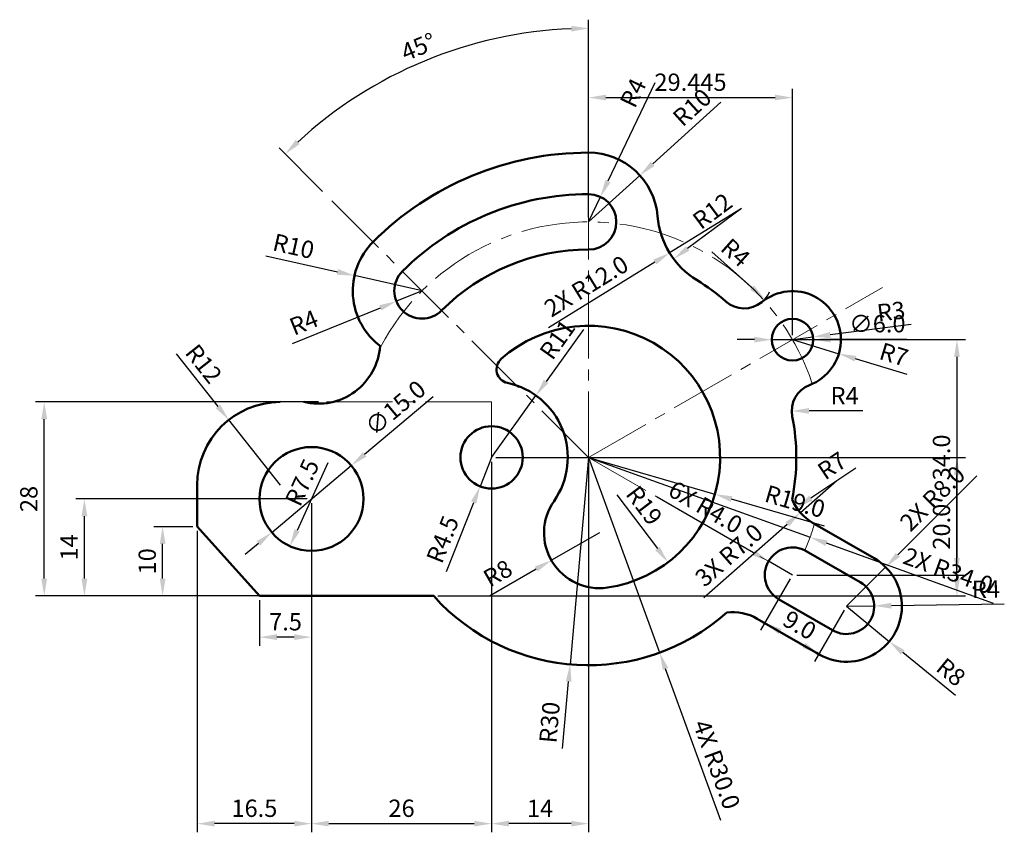
# Model space of a CAD drawing. Units: millimetres. Extents: x 1693 to 1835, y 1183 to 1300.
import ezdxf

# ---------------------------------------------------------------- set-up
doc = ezdxf.new("R2010")
doc.units = ezdxf.units.MM
doc.linetypes.add('CENTER2', pattern=[28.575, 19.05, -3.175, 3.175, -3.175])
for name, color, linetype, lineweight in [('M-CNTR', 4, 'CENTER2', 18), ('M-DIMS', 2, 'Continuous', 25), ('M-OUTL', 7, 'Continuous', 50)]:
    doc.layers.add(name, color=color, linetype=linetype, lineweight=lineweight)
doc.styles.get("Standard").update_dxf_attribs({"font": 'arial.ttf'})
doc.dimstyles.new('ISO-25', dxfattribs={"dimtxt": 2.5, "dimasz": 2.5, "dimexe": 1.25, "dimexo": 0.625, "dimtad": 1, "dimdsep": 46, "dimtxsty": 'Standard', "dimcen": 2.5, "dimadec": 0, "dimazin": 0, "dimtfac": 1, "dimtmove": 0, "dimatfit": 3, "dimfxl": 1, "dimarcsym": 0})

# ---------------------------------------------------------------- blocks, each defined once
blk = doc.blocks.new('*D1')
at = {"layer": 'Defpoints', "color": 0, "ltscale": 0.5, "transparency": 16777216}
for p in [(1759.38, 1296.69), (1775.41, 1275.52), (1737.44, 1274.82), (1775.41, 1236.85), (1775.41, 1236.85)]:
    blk.add_point(p, dxfattribs=at)
at = {"layer": 'M-DIMS', "color": 0, "lineweight": -2, "ltscale": 0.5, "transparency": 16777216}
for p, q in [((1775.41, 1276.15), (1775.41, 1300.05)), ((1737, 1275.26), (1730.72, 1281.54))]:
    blk.add_line(p, q, dxfattribs=at)
blk.add_arc((1775.41, 1236.85), 61.94, 92.3125, 132.6875, dxfattribs=at)
at = {"layer": 'M-DIMS', "color": 0, "ltscale": 0.5, "transparency": 16777216}
for points in [[(1772.9, 1299.16), (1772.92, 1298.33), (1775.41, 1298.8)], [(1733.7, 1282.09), (1733.12, 1282.69), (1731.61, 1280.65)]]:
    blk.add_solid(points, dxfattribs=at)
at = {"layer": 'M-DIMS', "color": 0, "ltscale": 0.5, "transparency": 16777216, "insert": (1750.98, 1295.83), "char_height": 2.5, "attachment_point": 5, "rotation": 22.5}
blk.add_mtext('45°', dxfattribs=at)
blk = doc.blocks.new('*D2')
at = {"layer": 'Defpoints', "color": 0, "transparency": 16777216}
for p in [(1777.13, 1274.46), (1775.41, 1270.85)]:
    blk.add_point(p, dxfattribs=at)
at = {"layer": 'M-DIMS', "color": 0, "lineweight": -2, "transparency": 16777216}
for p, q in [((1784.96, 1290.92), (1778.2, 1276.72)), ((1775.41, 1270.85), (1777.13, 1274.46))]:
    blk.add_line(p, q, dxfattribs=at)
at = {"layer": 'M-DIMS', "color": 0, "transparency": 16777216}
blk.add_solid([(1777.83, 1276.9), (1778.58, 1276.54), (1777.13, 1274.46)], dxfattribs=at)
at = {"layer": 'M-DIMS', "color": 0, "transparency": 16777216, "insert": (1782.13, 1289.34), "char_height": 2.5, "attachment_point": 5, "rotation": 64.5408}
blk.add_mtext('R4', dxfattribs=at)
blk = doc.blocks.new('*D3')
at = {"layer": 'Defpoints', "color": 0, "transparency": 16777216}
for p in [(1782.82, 1277.57), (1775.41, 1270.85)]:
    blk.add_point(p, dxfattribs=at)
at = {"layer": 'M-DIMS', "color": 0, "lineweight": -2, "transparency": 16777216}
for p, q in [((1794.52, 1288.16), (1784.67, 1279.24)), ((1775.41, 1270.85), (1782.82, 1277.57))]:
    blk.add_line(p, q, dxfattribs=at)
at = {"layer": 'M-DIMS', "color": 0, "transparency": 16777216}
blk.add_solid([(1784.39, 1279.55), (1784.95, 1278.93), (1782.82, 1277.57)], dxfattribs=at)
at = {"layer": 'M-DIMS', "color": 0, "transparency": 16777216, "insert": (1790.57, 1287.15), "char_height": 2.5, "attachment_point": 5, "rotation": 42.1642}
blk.add_mtext('R10', dxfattribs=at)
blk = doc.blocks.new('*D4')
at = {"layer": 'Defpoints', "color": 0, "transparency": 16777216}
for p in [(1804.85, 1253.85), (1811.55, 1251.82)]:
    blk.add_point(p, dxfattribs=at)
at = {"layer": 'M-DIMS', "color": 0, "lineweight": -2, "transparency": 16777216}
for p, q in [((1804.85, 1253.85), (1811.55, 1251.82)), ((1821.39, 1248.84), (1813.94, 1251.1))]:
    blk.add_line(p, q, dxfattribs=at)
at = {"layer": 'M-DIMS', "color": 0, "transparency": 16777216}
blk.add_solid([(1814.07, 1251.5), (1813.82, 1250.7), (1811.55, 1251.82)], dxfattribs=at)
at = {"layer": 'M-DIMS', "color": 0, "transparency": 16777216, "insert": (1819.41, 1251.4), "char_height": 2.5, "attachment_point": 5, "rotation": 343.1414}
blk.add_mtext('R7', dxfattribs=at)
blk = doc.blocks.new('*D5')
at = {"layer": 'Defpoints', "color": 0, "transparency": 16777216}
for p in [(1807.83, 1254.24), (1804.85, 1253.85)]:
    blk.add_point(p, dxfattribs=at)
at = {"layer": 'M-DIMS', "color": 0, "lineweight": -2, "transparency": 16777216}
for p, q in [((1821.99, 1256.06), (1810.31, 1254.56)), ((1804.85, 1253.85), (1807.83, 1254.24))]:
    blk.add_line(p, q, dxfattribs=at)
at = {"layer": 'M-DIMS', "color": 0, "transparency": 16777216}
blk.add_solid([(1810.25, 1254.97), (1810.36, 1254.14), (1807.83, 1254.24)], dxfattribs=at)
at = {"layer": 'M-DIMS', "color": 0, "transparency": 16777216, "insert": (1819.13, 1257.61), "char_height": 2.5, "attachment_point": 5, "rotation": 7.341}
blk.add_mtext('R3', dxfattribs=at)
blk = doc.blocks.new('*D6')
at = {"layer": 'Defpoints', "color": 0, "transparency": 16777216}
for p in [(1797.33, 1272.68), (1787.7, 1265.51)]:
    blk.add_point(p, dxfattribs=at)
at = {"layer": 'M-DIMS', "color": 0, "lineweight": -2, "transparency": 16777216}
blk.add_line((1797.49, 1272.79), (1789.71, 1267.01), dxfattribs=at)
at = {"layer": 'M-DIMS', "color": 0, "transparency": 16777216}
blk.add_solid([(1789.46, 1267.34), (1789.96, 1266.67), (1787.7, 1265.51)], dxfattribs=at)
at = {"layer": 'M-DIMS', "color": 0, "transparency": 16777216, "insert": (1793.48, 1272.16), "char_height": 2.5, "attachment_point": 5, "rotation": 36.6408}
blk.add_mtext('R12', dxfattribs=at)
blk = doc.blocks.new('*D7')
at = {"layer": 'Defpoints', "color": 0, "transparency": 16777216}
for p in [(1797.88, 1262.36), (1800.87, 1259.7)]:
    blk.add_point(p, dxfattribs=at)
at = {"layer": 'M-DIMS', "color": 0, "lineweight": -2, "transparency": 16777216}
blk.add_line((1793.21, 1266.54), (1799, 1261.36), dxfattribs=at)
blk.add_arc((1797.88, 1262.36), 4, 309.3093, 336.1142, dxfattribs=at)
at = {"layer": 'M-DIMS', "color": 0, "transparency": 16777216}
blk.add_solid([(1799.28, 1261.67), (1798.73, 1261.05), (1800.87, 1259.7)], dxfattribs=at)
at = {"layer": 'M-DIMS', "color": 0, "transparency": 16777216, "insert": (1796.42, 1266.18), "char_height": 2.5, "attachment_point": 5, "rotation": 318.2093}
blk.add_mtext('R4', dxfattribs=at)
blk = doc.blocks.new('*D8')
at = {"layer": 'Defpoints', "color": 0, "transparency": 16777216}
for p in [(1804.74, 1243.56), (1808.74, 1243.56)]:
    blk.add_point(p, dxfattribs=at)
at = {"layer": 'M-DIMS', "color": 0, "lineweight": -2, "transparency": 16777216}
blk.add_line((1815.01, 1243.56), (1807.24, 1243.56), dxfattribs=at)
at = {"layer": 'M-DIMS', "color": 0, "transparency": 16777216}
blk.add_solid([(1807.24, 1243.98), (1807.24, 1243.15), (1804.74, 1243.56)], dxfattribs=at)
at = {"layer": 'M-DIMS', "color": 0, "transparency": 16777216, "insert": (1812.38, 1245.44), "char_height": 2.5, "attachment_point": 5}
blk.add_mtext('R4', dxfattribs=at)
blk = doc.blocks.new('*D9')
at = {"layer": 'Defpoints', "color": 0, "transparency": 16777216}
for p in [(1811.25, 1233.48), (1805.44, 1229.58)]:
    blk.add_point(p, dxfattribs=at)
at = {"layer": 'M-DIMS', "color": 0, "lineweight": -2, "transparency": 16777216}
blk.add_line((1813.98, 1235.31), (1807.51, 1230.97), dxfattribs=at)
at = {"layer": 'M-DIMS', "color": 0, "transparency": 16777216}
blk.add_solid([(1807.28, 1231.32), (1807.74, 1230.63), (1805.44, 1229.58)], dxfattribs=at)
at = {"layer": 'M-DIMS', "color": 0, "transparency": 16777216, "insert": (1810.74, 1235.39), "char_height": 2.5, "attachment_point": 5, "rotation": 33.8392}
blk.add_mtext('R7', dxfattribs=at)
blk = doc.blocks.new('*D10')
at = {"layer": 'Defpoints', "color": 0, "transparency": 16777216}
for p in [(1812.65, 1215.35), (1816.65, 1215.41)]:
    blk.add_point(p, dxfattribs=at)
at = {"layer": 'M-DIMS', "color": 0, "lineweight": -2, "transparency": 16777216}
for p, q in [((1835.44, 1215.66), (1819.15, 1215.44)), ((1812.65, 1215.35), (1816.65, 1215.41))]:
    blk.add_line(p, q, dxfattribs=at)
at = {"layer": 'M-DIMS', "color": 0, "transparency": 16777216}
blk.add_solid([(1819.14, 1215.86), (1819.15, 1215.02), (1816.65, 1215.41)], dxfattribs=at)
at = {"layer": 'M-DIMS', "color": 0, "transparency": 16777216, "insert": (1832.78, 1217.5), "char_height": 2.5, "attachment_point": 5, "rotation": 0.7634}
blk.add_mtext('R4', dxfattribs=at)
blk = doc.blocks.new('*D11')
at = {"layer": 'Defpoints', "color": 0, "transparency": 16777216}
for p in [(1812.65, 1215.35), (1818.83, 1210.28)]:
    blk.add_point(p, dxfattribs=at)
at = {"layer": 'M-DIMS', "color": 0, "lineweight": -2, "transparency": 16777216}
for p, q in [((1812.65, 1215.35), (1818.83, 1210.28)), ((1828.37, 1202.46), (1820.77, 1208.7))]:
    blk.add_line(p, q, dxfattribs=at)
at = {"layer": 'M-DIMS', "color": 0, "transparency": 16777216}
blk.add_solid([(1821.03, 1209.02), (1820.5, 1208.37), (1818.83, 1210.28)], dxfattribs=at)
at = {"layer": 'M-DIMS', "color": 0, "transparency": 16777216, "insert": (1827.54, 1205.61), "char_height": 2.5, "attachment_point": 5, "rotation": 320.6579}
blk.add_mtext('R8', dxfattribs=at)
blk = doc.blocks.new('*D12')
at = {"layer": 'Defpoints', "color": 0, "transparency": 16777216}
for p in [(1775.41, 1236.85), (1772.75, 1206.97)]:
    blk.add_point(p, dxfattribs=at)
at = {"layer": 'M-DIMS', "color": 0, "lineweight": -2, "transparency": 16777216}
for p, q in [((1775.41, 1236.85), (1772.75, 1206.97)), ((1771.67, 1194.8), (1772.53, 1204.48))]:
    blk.add_line(p, q, dxfattribs=at)
at = {"layer": 'M-DIMS', "color": 0, "transparency": 16777216}
blk.add_solid([(1772.12, 1204.52), (1772.95, 1204.44), (1772.75, 1206.97)], dxfattribs=at)
at = {"layer": 'M-DIMS', "color": 0, "transparency": 16777216, "insert": (1770.1, 1198.56), "char_height": 2.5, "attachment_point": 5, "rotation": 84.925}
blk.add_mtext('R30', dxfattribs=at)
blk = doc.blocks.new('*D13')
at = {"layer": 'Defpoints', "color": 0, "transparency": 16777216}
for p in [(1775.41, 1236.85), (1786.87, 1221.7)]:
    blk.add_point(p, dxfattribs=at)
at = {"layer": 'M-DIMS', "color": 0, "lineweight": -2, "transparency": 16777216}
blk.add_line((1779.49, 1231.45), (1785.36, 1223.69), dxfattribs=at)
at = {"layer": 'M-DIMS', "color": 0, "transparency": 16777216}
blk.add_solid([(1785.69, 1223.94), (1785.03, 1223.44), (1786.87, 1221.7)], dxfattribs=at)
at = {"layer": 'M-DIMS', "color": 0, "transparency": 16777216, "insert": (1783.19, 1229.72), "char_height": 2.5, "attachment_point": 5, "rotation": 307.0947}
blk.add_mtext('R19', dxfattribs=at)
blk = doc.blocks.new('*D14')
at = {"layer": 'Defpoints', "color": 0, "transparency": 16777216}
for p in [(1767.82, 1245.79), (1761.41, 1236.85)]:
    blk.add_point(p, dxfattribs=at)
at = {"layer": 'M-DIMS', "color": 0, "lineweight": -2, "transparency": 16777216}
for p, q in [((1774.66, 1255.33), (1769.27, 1247.82)), ((1761.41, 1236.85), (1767.82, 1245.79))]:
    blk.add_line(p, q, dxfattribs=at)
at = {"layer": 'M-DIMS', "color": 0, "transparency": 16777216}
blk.add_solid([(1768.94, 1248.07), (1769.61, 1247.58), (1767.82, 1245.79)], dxfattribs=at)
at = {"layer": 'M-DIMS', "color": 0, "transparency": 16777216, "insert": (1771.17, 1253.69), "char_height": 2.5, "attachment_point": 5, "rotation": 54.359}
blk.add_mtext('R11', dxfattribs=at)
blk = doc.blocks.new('*D15')
at = {"layer": 'Defpoints', "color": 0, "transparency": 16777216}
for p in [(1776.98, 1225.97), (1770.04, 1221.99)]:
    blk.add_point(p, dxfattribs=at)
at = {"layer": 'M-DIMS', "color": 0, "lineweight": -2, "transparency": 16777216}
for p, q in [((1776.98, 1225.97), (1770.04, 1221.99)), ((1761.11, 1216.88), (1767.87, 1220.75))]:
    blk.add_line(p, q, dxfattribs=at)
at = {"layer": 'M-DIMS', "color": 0, "transparency": 16777216}
blk.add_solid([(1767.66, 1221.11), (1768.07, 1220.39), (1770.04, 1221.99)], dxfattribs=at)
at = {"layer": 'M-DIMS', "color": 0, "transparency": 16777216, "insert": (1762.46, 1219.85), "char_height": 2.5, "attachment_point": 5, "rotation": 29.7797}
blk.add_mtext('R8', dxfattribs=at)
blk = doc.blocks.new('*D16')
at = {"layer": 'Defpoints', "color": 0, "transparency": 16777216}
for p in [(1761.41, 1236.85), (1759.75, 1232.67)]:
    blk.add_point(p, dxfattribs=at)
at = {"layer": 'M-DIMS', "color": 0, "lineweight": -2, "transparency": 16777216}
for p, q in [((1761.41, 1236.85), (1759.75, 1232.67)), ((1754.89, 1220.38), (1758.83, 1230.34))]:
    blk.add_line(p, q, dxfattribs=at)
at = {"layer": 'M-DIMS', "color": 0, "transparency": 16777216}
blk.add_solid([(1758.44, 1230.5), (1759.22, 1230.19), (1759.75, 1232.67)], dxfattribs=at)
at = {"layer": 'M-DIMS', "color": 0, "transparency": 16777216, "insert": (1754.64, 1224.9), "char_height": 2.5, "attachment_point": 5, "rotation": 68.4068}
blk.add_mtext('R4.5', dxfattribs=at)
blk = doc.blocks.new('*D17')
at = {"layer": 'Defpoints', "color": 0, "transparency": 16777216}
for p in [(1735.41, 1230.85), (1732.28, 1224.03)]:
    blk.add_point(p, dxfattribs=at)
at = {"layer": 'M-DIMS', "color": 0, "lineweight": -2, "transparency": 16777216}
blk.add_line((1737.79, 1236.05), (1733.33, 1226.31), dxfattribs=at)
at = {"layer": 'M-DIMS', "color": 0, "transparency": 16777216}
blk.add_solid([(1732.95, 1226.48), (1733.7, 1226.13), (1732.28, 1224.03)], dxfattribs=at)
at = {"layer": 'M-DIMS', "color": 0, "transparency": 16777216, "insert": (1734.35, 1233.1), "char_height": 2.5, "attachment_point": 5, "rotation": 65.3962}
blk.add_mtext('R7.5', dxfattribs=at)
blk = doc.blocks.new('*D18')
at = {"layer": 'Defpoints', "color": 0, "transparency": 16777216}
for p in [(1723.46, 1242.26), (1730.91, 1232.85)]:
    blk.add_point(p, dxfattribs=at)
at = {"layer": 'M-DIMS', "color": 0, "lineweight": -2, "transparency": 16777216}
for p, q in [((1715.88, 1251.82), (1721.9, 1244.22)), ((1730.91, 1232.85), (1723.46, 1242.26))]:
    blk.add_line(p, q, dxfattribs=at)
at = {"layer": 'M-DIMS', "color": 0, "transparency": 16777216}
blk.add_solid([(1722.23, 1244.48), (1721.58, 1243.96), (1723.46, 1242.26)], dxfattribs=at)
at = {"layer": 'M-DIMS', "color": 0, "transparency": 16777216, "insert": (1719.59, 1250.17), "char_height": 2.5, "attachment_point": 5, "rotation": 308.3851}
blk.add_mtext('R12', dxfattribs=at)
blk = doc.blocks.new('*D19')
at = {"layer": 'Defpoints', "color": 0, "transparency": 16777216}
for p in [(1751.37, 1260.89), (1747.66, 1259.39)]:
    blk.add_point(p, dxfattribs=at)
at = {"layer": 'M-DIMS', "color": 0, "lineweight": -2, "transparency": 16777216}
for p, q in [((1751.37, 1260.89), (1747.66, 1259.39)), ((1732.68, 1253.29), (1745.35, 1258.44))]:
    blk.add_line(p, q, dxfattribs=at)
at = {"layer": 'M-DIMS', "color": 0, "transparency": 16777216}
blk.add_solid([(1745.19, 1258.83), (1745.5, 1258.06), (1747.66, 1259.39)], dxfattribs=at)
at = {"layer": 'M-DIMS', "color": 0, "transparency": 16777216, "insert": (1734.42, 1256.02), "char_height": 2.5, "attachment_point": 5, "rotation": 22.1456}
blk.add_mtext('R4', dxfattribs=at)
blk = doc.blocks.new('*D20')
at = {"layer": 'Defpoints', "color": 0, "transparency": 16777216}
for p in [(1741.61, 1263.09), (1751.37, 1260.89)]:
    blk.add_point(p, dxfattribs=at)
at = {"layer": 'M-DIMS', "color": 0, "lineweight": -2, "transparency": 16777216}
for p, q in [((1728.82, 1265.97), (1739.17, 1263.64)), ((1751.37, 1260.89), (1741.61, 1263.09))]:
    blk.add_line(p, q, dxfattribs=at)
at = {"layer": 'M-DIMS', "color": 0, "transparency": 16777216}
blk.add_solid([(1739.26, 1264.05), (1739.08, 1263.23), (1741.61, 1263.09)], dxfattribs=at)
at = {"layer": 'M-DIMS', "color": 0, "transparency": 16777216, "insert": (1732.75, 1267.03), "char_height": 2.5, "attachment_point": 5, "rotation": 347.3173}
blk.add_mtext('R10', dxfattribs=at)
blk = doc.blocks.new('*D21')
at = {"layer": 'Defpoints', "color": 0, "transparency": 16777216}
for p in [(1735.41, 1230.85), (1727.91, 1216.85), (1727.91, 1210.9)]:
    blk.add_point(p, dxfattribs=at)
at = {"layer": 'M-DIMS', "color": 0, "lineweight": -2, "transparency": 16777216}
for p, q in [((1735.41, 1230.23), (1735.41, 1209.65)), ((1727.91, 1216.23), (1727.91, 1209.65)), ((1732.91, 1210.9), (1730.41, 1210.9))]:
    blk.add_line(p, q, dxfattribs=at)
at = {"layer": 'M-DIMS', "color": 0, "transparency": 16777216}
for points in [[(1730.41, 1211.32), (1730.41, 1210.48), (1727.91, 1210.9)], [(1732.91, 1211.32), (1732.91, 1210.48), (1735.41, 1210.9)]]:
    blk.add_solid(points, dxfattribs=at)
at = {"layer": 'M-DIMS', "color": 0, "transparency": 16777216, "insert": (1731.66, 1212.8), "char_height": 2.5, "attachment_point": 5}
blk.add_mtext('7.5', dxfattribs=at)
blk = doc.blocks.new('*D22')
at = {"layer": 'Defpoints', "color": 0, "transparency": 16777216}
for p in [(1713.91, 1226.85), (1718.91, 1226.85), (1727.91, 1216.85)]:
    blk.add_point(p, dxfattribs=at)
at = {"layer": 'M-DIMS', "color": 0, "lineweight": -2, "transparency": 16777216}
for p, q in [((1718.28, 1226.85), (1712.66, 1226.85)), ((1713.91, 1219.35), (1713.91, 1224.35)), ((1727.28, 1216.85), (1712.66, 1216.85))]:
    blk.add_line(p, q, dxfattribs=at)
at = {"layer": 'M-DIMS', "color": 0, "transparency": 16777216}
for points in [[(1713.5, 1224.35), (1714.33, 1224.35), (1713.91, 1226.85)], [(1713.5, 1219.35), (1714.33, 1219.35), (1713.91, 1216.85)]]:
    blk.add_solid(points, dxfattribs=at)
at = {"layer": 'M-DIMS', "color": 0, "transparency": 16777216, "insert": (1712.01, 1221.85), "char_height": 2.5, "attachment_point": 5, "rotation": 90}
blk.add_mtext('10', dxfattribs=at)
blk = doc.blocks.new('*D23')
at = {"layer": 'Defpoints', "color": 0, "transparency": 16777216}
for p in [(1702.62, 1230.85), (1735.41, 1230.85), (1727.91, 1216.85)]:
    blk.add_point(p, dxfattribs=at)
at = {"layer": 'M-DIMS', "color": 0, "lineweight": -2, "transparency": 16777216}
for p, q in [((1734.78, 1230.85), (1701.37, 1230.85)), ((1702.62, 1219.35), (1702.62, 1228.35)), ((1727.28, 1216.85), (1701.37, 1216.85))]:
    blk.add_line(p, q, dxfattribs=at)
at = {"layer": 'M-DIMS', "color": 0, "transparency": 16777216}
for points in [[(1702.2, 1228.35), (1703.04, 1228.35), (1702.62, 1230.85)], [(1702.2, 1219.35), (1703.04, 1219.35), (1702.62, 1216.85)]]:
    blk.add_solid(points, dxfattribs=at)
at = {"layer": 'M-DIMS', "color": 0, "transparency": 16777216, "insert": (1700.74, 1223.85), "char_height": 2.5, "attachment_point": 5, "rotation": 90}
blk.add_mtext('14', dxfattribs=at)
blk = doc.blocks.new('*D24')
at = {"layer": 'Defpoints', "color": 0, "transparency": 16777216}
for p in [(1696.82, 1244.85), (1737.03, 1244.85), (1735.41, 1216.85)]:
    blk.add_point(p, dxfattribs=at)
at = {"layer": 'M-DIMS', "color": 0, "lineweight": -2, "transparency": 16777216}
for p, q in [((1736.4, 1244.85), (1695.57, 1244.85)), ((1696.82, 1219.35), (1696.82, 1242.35)), ((1734.78, 1216.85), (1695.57, 1216.85))]:
    blk.add_line(p, q, dxfattribs=at)
at = {"layer": 'M-DIMS', "color": 0, "transparency": 16777216}
for points in [[(1696.4, 1242.35), (1697.24, 1242.35), (1696.82, 1244.85)], [(1696.4, 1219.35), (1697.24, 1219.35), (1696.82, 1216.85)]]:
    blk.add_solid(points, dxfattribs=at)
at = {"layer": 'M-DIMS', "color": 0, "transparency": 16777216, "insert": (1694.92, 1230.85), "char_height": 2.5, "attachment_point": 5, "rotation": 90}
blk.add_mtext('28', dxfattribs=at)
blk = doc.blocks.new('*D25')
at = {"layer": 'Defpoints', "color": 0, "transparency": 16777216}
for p in [(1735.41, 1230.85), (1718.91, 1226.85), (1718.91, 1183.97)]:
    blk.add_point(p, dxfattribs=at)
at = {"layer": 'M-DIMS', "color": 0, "lineweight": -2, "transparency": 16777216}
for p, q in [((1735.41, 1230.23), (1735.41, 1182.72)), ((1718.91, 1226.23), (1718.91, 1182.72)), ((1732.91, 1183.97), (1721.41, 1183.97))]:
    blk.add_line(p, q, dxfattribs=at)
at = {"layer": 'M-DIMS', "color": 0, "transparency": 16777216}
for points in [[(1721.41, 1184.39), (1721.41, 1183.56), (1718.91, 1183.97)], [(1732.91, 1184.39), (1732.91, 1183.56), (1735.41, 1183.97)]]:
    blk.add_solid(points, dxfattribs=at)
at = {"layer": 'M-DIMS', "color": 0, "transparency": 16777216, "insert": (1727.16, 1185.87), "char_height": 2.5, "attachment_point": 5}
blk.add_mtext('16.5', dxfattribs=at)
blk = doc.blocks.new('*D26')
at = {"layer": 'Defpoints', "color": 0, "transparency": 16777216}
for p in [(1761.41, 1236.85), (1735.41, 1230.85), (1761.41, 1183.97)]:
    blk.add_point(p, dxfattribs=at)
at = {"layer": 'M-DIMS', "color": 0, "lineweight": -2, "transparency": 16777216}
for p, q in [((1761.41, 1236.23), (1761.41, 1182.72)), ((1735.41, 1230.23), (1735.41, 1182.72)), ((1737.91, 1183.97), (1758.91, 1183.97))]:
    blk.add_line(p, q, dxfattribs=at)
at = {"layer": 'M-DIMS', "color": 0, "transparency": 16777216}
for points in [[(1737.91, 1184.39), (1737.91, 1183.56), (1735.41, 1183.97)], [(1758.91, 1184.39), (1758.91, 1183.56), (1761.41, 1183.97)]]:
    blk.add_solid(points, dxfattribs=at)
at = {"layer": 'M-DIMS', "color": 0, "transparency": 16777216, "insert": (1748.41, 1185.87), "char_height": 2.5, "attachment_point": 5}
blk.add_mtext('26', dxfattribs=at)
blk = doc.blocks.new('*D27')
at = {"layer": 'Defpoints', "color": 0, "transparency": 16777216}
for p in [(1761.41, 1236.85), (1775.41, 1236.85), (1761.41, 1183.97)]:
    blk.add_point(p, dxfattribs=at)
at = {"layer": 'M-DIMS', "color": 0, "lineweight": -2, "transparency": 16777216}
for p, q in [((1761.41, 1236.23), (1761.41, 1182.72)), ((1775.41, 1236.23), (1775.41, 1182.72)), ((1772.91, 1183.97), (1763.91, 1183.97))]:
    blk.add_line(p, q, dxfattribs=at)
at = {"layer": 'M-DIMS', "color": 0, "transparency": 16777216}
for points in [[(1763.91, 1184.39), (1763.91, 1183.56), (1761.41, 1183.97)], [(1772.91, 1184.39), (1772.91, 1183.56), (1775.41, 1183.97)]]:
    blk.add_solid(points, dxfattribs=at)
at = {"layer": 'M-DIMS', "color": 0, "transparency": 16777216, "insert": (1768.41, 1185.85), "char_height": 2.5, "attachment_point": 5}
blk.add_mtext('14', dxfattribs=at)
blk = doc.blocks.new('*D28')
at = {"layer": 'Defpoints', "color": 0, "transparency": 16777216}
for p in [(1761.41, 1236.85), (1828.6, 1236.85), (1753.05, 1216.85)]:
    blk.add_point(p, dxfattribs=at)
at = {"layer": 'M-DIMS', "color": 0, "lineweight": -2, "transparency": 16777216}
for p, q in [((1762.03, 1236.85), (1829.85, 1236.85)), ((1828.6, 1219.35), (1828.6, 1234.35)), ((1753.67, 1216.85), (1829.85, 1216.85))]:
    blk.add_line(p, q, dxfattribs=at)
at = {"layer": 'M-DIMS', "color": 0, "transparency": 16777216}
for points in [[(1828.18, 1234.35), (1829.01, 1234.35), (1828.6, 1236.85)], [(1828.18, 1219.35), (1829.01, 1219.35), (1828.6, 1216.85)]]:
    blk.add_solid(points, dxfattribs=at)
at = {"layer": 'M-DIMS', "color": 0, "transparency": 16777216, "insert": (1826.69, 1226.85), "char_height": 2.5, "attachment_point": 5, "rotation": 90}
blk.add_mtext('20.0', dxfattribs=at)
blk = doc.blocks.new('*D29')
at = {"layer": 'Defpoints', "color": 0, "transparency": 16777216}
for p in [(1804.85, 1219.85), (1812.65, 1215.35), (1800.88, 1212.97)]:
    blk.add_point(p, dxfattribs=at)
at = {"layer": 'M-DIMS', "color": 0, "lineweight": -2, "transparency": 16777216}
for p, q in [((1804.54, 1219.31), (1800.25, 1211.89)), ((1812.33, 1214.81), (1808.05, 1207.39)), ((1806.51, 1209.72), (1803.04, 1211.72))]:
    blk.add_line(p, q, dxfattribs=at)
at = {"layer": 'M-DIMS', "color": 0, "transparency": 16777216}
for points in [[(1803.25, 1212.08), (1802.83, 1211.36), (1800.88, 1212.97)], [(1806.72, 1210.08), (1806.3, 1209.36), (1808.67, 1208.47)]]:
    blk.add_solid(points, dxfattribs=at)
at = {"layer": 'M-DIMS', "color": 0, "transparency": 16777216, "insert": (1805.73, 1212.36), "char_height": 2.5, "attachment_point": 5, "rotation": 330}
blk.add_mtext('9.0', dxfattribs=at)
blk = doc.blocks.new('*D30')
at = {"layer": 'Defpoints', "color": 0, "transparency": 16777216}
for p in [(1804.85, 1253.85), (1804.85, 1219.85), (1828.6, 1219.85)]:
    blk.add_point(p, dxfattribs=at)
at = {"layer": 'M-DIMS', "color": 0, "lineweight": -2, "transparency": 16777216}
for p, q in [((1805.48, 1253.85), (1829.85, 1253.85)), ((1828.6, 1251.35), (1828.6, 1222.35)), ((1805.48, 1219.85), (1829.85, 1219.85))]:
    blk.add_line(p, q, dxfattribs=at)
at = {"layer": 'M-DIMS', "color": 0, "transparency": 16777216}
for points in [[(1828.18, 1251.35), (1829.01, 1251.35), (1828.6, 1253.85)], [(1828.18, 1222.35), (1829.01, 1222.35), (1828.6, 1219.85)]]:
    blk.add_solid(points, dxfattribs=at)
at = {"layer": 'M-DIMS', "color": 0, "transparency": 16777216, "insert": (1826.69, 1236.85), "char_height": 2.5, "attachment_point": 5, "rotation": 90}
blk.add_mtext('34.0', dxfattribs=at)
blk = doc.blocks.new('*D31')
at = {"layer": 'Defpoints', "color": 0, "transparency": 16777216}
for p in [(1804.85, 1288.8), (1775.41, 1270.85), (1804.85, 1253.85)]:
    blk.add_point(p, dxfattribs=at)
at = {"layer": 'M-DIMS', "color": 0, "lineweight": -2, "transparency": 16777216}
for p, q in [((1775.41, 1271.48), (1775.41, 1290.05)), ((1804.85, 1254.48), (1804.85, 1290.05)), ((1777.91, 1288.8), (1802.35, 1288.8))]:
    blk.add_line(p, q, dxfattribs=at)
at = {"layer": 'M-DIMS', "color": 0, "transparency": 16777216}
for points in [[(1777.91, 1289.22), (1777.91, 1288.39), (1775.41, 1288.8)], [(1802.35, 1289.22), (1802.35, 1288.39), (1804.85, 1288.8)]]:
    blk.add_solid(points, dxfattribs=at)
at = {"layer": 'M-DIMS', "color": 0, "transparency": 16777216, "insert": (1790.13, 1290.7), "char_height": 2.5, "attachment_point": 5}
blk.add_mtext('29.445', dxfattribs=at)
blk = doc.blocks.new('*D32')
at = {"layer": 'Defpoints', "color": 0, "transparency": 16777216}
for p in [(1775.41, 1236.85), (1807.39, 1225.32)]:
    blk.add_point(p, dxfattribs=at)
at = {"layer": 'M-DIMS', "color": 0, "lineweight": -2, "transparency": 16777216}
for p, q in [((1775.41, 1236.85), (1807.39, 1225.32)), ((1833.9, 1215.77), (1809.75, 1224.48))]:
    blk.add_line(p, q, dxfattribs=at)
at = {"layer": 'M-DIMS', "color": 0, "transparency": 16777216}
blk.add_solid([(1809.89, 1224.87), (1809.6, 1224.08), (1807.39, 1225.32)], dxfattribs=at)
at = {"layer": 'M-DIMS', "color": 0, "transparency": 16777216, "insert": (1827.23, 1220.19), "char_height": 2.5, "attachment_point": 5, "rotation": 340.1778}
blk.add_mtext('2X R34.0', dxfattribs=at)
blk = doc.blocks.new('*D33')
at = {"layer": 'Defpoints', "color": 0, "transparency": 16777216}
for p in [(1775.41, 1236.85), (1785.67, 1208.66)]:
    blk.add_point(p, dxfattribs=at)
at = {"layer": 'M-DIMS', "color": 0, "lineweight": -2, "transparency": 16777216}
for p, q in [((1775.41, 1236.85), (1785.67, 1208.66)), ((1794.49, 1184.42), (1786.52, 1206.31))]:
    blk.add_line(p, q, dxfattribs=at)
at = {"layer": 'M-DIMS', "color": 0, "transparency": 16777216}
blk.add_solid([(1786.92, 1206.46), (1786.13, 1206.17), (1785.67, 1208.66)], dxfattribs=at)
at = {"layer": 'M-DIMS', "color": 0, "transparency": 16777216, "insert": (1793.61, 1192.4), "char_height": 2.5, "attachment_point": 5, "rotation": 290.0003}
blk.add_mtext('4X R30.0', dxfattribs=at)
blk = doc.blocks.new('*D34')
at = {"layer": 'Defpoints', "color": 0, "transparency": 16777216}
for p in [(1775.41, 1236.85), (1793.65, 1231.54)]:
    blk.add_point(p, dxfattribs=at)
at = {"layer": 'M-DIMS', "color": 0, "lineweight": -2, "transparency": 16777216}
for p, q in [((1775.41, 1236.85), (1793.65, 1231.54)), ((1809.46, 1226.94), (1796.05, 1230.84))]:
    blk.add_line(p, q, dxfattribs=at)
at = {"layer": 'M-DIMS', "color": 0, "transparency": 16777216}
blk.add_solid([(1796.17, 1231.24), (1795.93, 1230.44), (1793.65, 1231.54)], dxfattribs=at)
at = {"layer": 'M-DIMS', "color": 0, "transparency": 16777216, "insert": (1805.13, 1230.18), "char_height": 2.5, "attachment_point": 5, "rotation": 343.7627}
blk.add_mtext('R19.0', dxfattribs=at)
blk = doc.blocks.new('*D35')
at = {"layer": 'Defpoints', "color": 0, "transparency": 16777216}
for p in [(1797.33, 1272.68), (1787.12, 1266.38)]:
    blk.add_point(p, dxfattribs=at)
at = {"layer": 'M-DIMS', "color": 0, "lineweight": -2, "transparency": 16777216}
for p, q in [((1797.33, 1272.68), (1787.12, 1266.38)), ((1769.63, 1255.6), (1784.99, 1265.07))]:
    blk.add_line(p, q, dxfattribs=at)
at = {"layer": 'M-DIMS', "color": 0, "transparency": 16777216}
blk.add_solid([(1784.77, 1265.42), (1785.21, 1264.71), (1787.12, 1266.38)], dxfattribs=at)
at = {"layer": 'M-DIMS', "color": 0, "transparency": 16777216, "insert": (1775.25, 1261.3), "char_height": 2.5, "attachment_point": 5, "rotation": 31.6465}
blk.add_mtext('2X R12.0', dxfattribs=at)
blk = doc.blocks.new('*D36')
at = {"layer": 'Defpoints', "color": 0, "transparency": 16777216}
for p in [(1818.3, 1221.01), (1812.65, 1215.35)]:
    blk.add_point(p, dxfattribs=at)
at = {"layer": 'M-DIMS', "color": 0, "lineweight": -2, "transparency": 16777216}
for p, q in [((1831.45, 1234.17), (1820.07, 1222.78)), ((1812.65, 1215.35), (1818.3, 1221.01))]:
    blk.add_line(p, q, dxfattribs=at)
at = {"layer": 'M-DIMS', "color": 0, "transparency": 16777216}
blk.add_solid([(1819.77, 1223.07), (1820.36, 1222.49), (1818.3, 1221.01)], dxfattribs=at)
at = {"layer": 'M-DIMS', "color": 0, "transparency": 16777216, "insert": (1825.3, 1230.7), "char_height": 2.5, "attachment_point": 5, "rotation": 45.0244}
blk.add_mtext('2X R8.0', dxfattribs=at)
blk = doc.blocks.new('*D37')
at = {"layer": 'Defpoints', "color": 0, "transparency": 16777216}
for p in [(1741.15, 1235.67), (1729.66, 1226.03)]:
    blk.add_point(p, dxfattribs=at)
at = {"layer": 'M-DIMS', "color": 0, "lineweight": -2, "transparency": 16777216}
for p, q in [((1752.99, 1245.6), (1743.07, 1237.28)), ((1729.66, 1226.03), (1741.15, 1235.67)), ((1727.75, 1224.43), (1725.83, 1222.82))]:
    blk.add_line(p, q, dxfattribs=at)
at = {"layer": 'M-DIMS', "color": 0, "transparency": 16777216}
for points in [[(1742.8, 1237.6), (1743.34, 1236.96), (1741.15, 1235.67)], [(1727.48, 1224.75), (1728.01, 1224.11), (1729.66, 1226.03)]]:
    blk.add_solid(points, dxfattribs=at)
at = {"layer": 'M-DIMS', "color": 0, "transparency": 16777216, "insert": (1747.72, 1243.76), "char_height": 2.5, "attachment_point": 5, "rotation": 39.9901}
blk.add_mtext('∅15.0', dxfattribs=at)
blk = doc.blocks.new('*D38')
at = {"layer": 'Defpoints', "color": 0, "transparency": 16777216}
for p in [(1811.25, 1233.48), (1805.99, 1228.86)]:
    blk.add_point(p, dxfattribs=at)
at = {"layer": 'M-DIMS', "color": 0, "lineweight": -2, "transparency": 16777216}
for p, q in [((1811.25, 1233.48), (1805.99, 1228.86)), ((1792.05, 1216.61), (1804.11, 1227.21))]:
    blk.add_line(p, q, dxfattribs=at)
at = {"layer": 'M-DIMS', "color": 0, "transparency": 16777216}
blk.add_solid([(1803.84, 1227.52), (1804.39, 1226.9), (1805.99, 1228.86)], dxfattribs=at)
at = {"layer": 'M-DIMS', "color": 0, "transparency": 16777216, "insert": (1795.89, 1222.51), "char_height": 2.5, "attachment_point": 5, "rotation": 41.3102}
blk.add_mtext('3X R7.0', dxfattribs=at)
blk = doc.blocks.new('*D39')
at = {"layer": 'Defpoints', "color": 0, "transparency": 16777216}
for p in [(1801.39, 1221.85), (1804.85, 1219.85)]:
    blk.add_point(p, dxfattribs=at)
at = {"layer": 'M-DIMS', "color": 0, "lineweight": -2, "transparency": 16777216}
for p, q in [((1785.31, 1231.14), (1799.22, 1223.1)), ((1804.85, 1219.85), (1801.39, 1221.85))]:
    blk.add_line(p, q, dxfattribs=at)
at = {"layer": 'M-DIMS', "color": 0, "transparency": 16777216}
blk.add_solid([(1799.43, 1223.46), (1799.02, 1222.74), (1801.39, 1221.85)], dxfattribs=at)
at = {"layer": 'M-DIMS', "color": 0, "transparency": 16777216, "insert": (1792.13, 1229.39), "char_height": 2.5, "attachment_point": 5, "rotation": 329.9952}
blk.add_mtext('6X R4.0', dxfattribs=at)
blk = doc.blocks.new('*D40')
at = {"layer": 'Defpoints', "color": 0, "transparency": 16777216}
for p in [(1801.85, 1253.85), (1807.85, 1253.85)]:
    blk.add_point(p, dxfattribs=at)
at = {"layer": 'M-DIMS', "color": 0, "lineweight": -2, "transparency": 16777216}
for p, q in [((1821.37, 1253.85), (1810.35, 1253.85)), ((1799.35, 1253.85), (1796.85, 1253.85)), ((1801.85, 1253.85), (1807.85, 1253.85))]:
    blk.add_line(p, q, dxfattribs=at)
at = {"layer": 'M-DIMS', "color": 0, "transparency": 16777216}
for points in [[(1799.35, 1254.27), (1799.35, 1253.44), (1801.85, 1253.85)], [(1810.35, 1254.27), (1810.35, 1253.44), (1807.85, 1253.85)]]:
    blk.add_solid(points, dxfattribs=at)
at = {"layer": 'M-DIMS', "color": 0, "transparency": 16777216, "insert": (1817.11, 1255.83), "char_height": 2.5, "attachment_point": 5, "rotation": 0.0081}
blk.add_mtext('∅6.0', dxfattribs=at)

msp = doc.modelspace()

# ---------------------------------------------------------------- linework, layer by layer
at = {"layer": 'M-CNTR', "ltscale": 0.5}
for p, q in [((1775.4083, 1236.8526), (1775.4083, 1275.5237)), ((1775.4083, 1236.8526), (1737.4434, 1274.8175)), ((1775.4083, 1236.8526), (1817.8658, 1261.3654)), ((1761.4083, 1244.8526), (1730.9068, 1244.8526)), ((1761.4083, 1236.8526), (1761.4083, 1244.8526)), ((1775.4083, 1236.8526), (1761.4083, 1236.8526)), ((1775.4083, 1236.8526), (1801.3891, 1221.8526))]:
    msp.add_line(p, q, dxfattribs=at)
for start, end in [(18.182874, 151.91727), (336.744573, 343.608961)]:
    msp.add_arc((1775.4083, 1236.8526), 34, start, end, dxfattribs=at)
at = {"layer": 'M-OUTL'}
for p, q in [((1718.9068, 1226.8526), (1718.9068, 1232.8526)), ((1727.9068, 1216.8526), (1718.9068, 1226.8526)), ((1807.75, 1227.4177), (1816.6474, 1222.2808)), ((1806.8532, 1223.3167), (1814.6474, 1218.8167)), ((1753.0476, 1216.8526), (1727.9068, 1216.8526)), ((1802.8532, 1216.3885), (1810.6474, 1211.8885)), ((1799.7584, 1213.5673), (1808.8893, 1208.2956))]:
    msp.add_line(p, q, dxfattribs=at)
for centre, radius in [((1804.8532, 1253.8526), 3), ((1761.4083, 1236.8526), 4.5), ((1735.4068, 1230.8526), 7.5)]:
    msp.add_circle(centre, radius, dxfattribs=at)
for centre, radius, start, end in [((1775.4083, 1236.8526), 44, 90, 135), ((1775.4083, 1270.8526), 10, 4.75457, 90), ((1775.4083, 1236.8526), 38, 90, 135), ((1775.4083, 1270.8526), 4, 270, 90), ((1797.3326, 1272.6761), 12, 184.75457, 238.533024), ((1751.3667, 1260.8942), 10, 135, 233.456519), ((1775.4083, 1236.8526), 30, 90, 135), ((1751.3667, 1260.8942), 4, 135, 315), ((1775.4083, 1236.8526), 30, 48.61868, 58.533024), ((1804.8532, 1253.8526), 7, 290.690656, 129.30934), ((1797.8846, 1262.3637), 4, 228.61868, 309.30934), ((1775.4083, 1236.8526), 19, 278.213211, 131.595352), ((1736.3816, 1253.5629), 8.9538, 256.452741, 355.975327), ((1764.1226, 1249.5661), 2, 131.595352, 257.948477), ((1761.4083, 1236.8526), 11, 325.03966, 77.948477), ((1808.7397, 1243.5621), 4, 110.690656, 191.381316), ((1730.9068, 1232.8526), 12, 90, 180), ((1775.4083, 1236.8526), 30, 348.335045, 11.381316), ((1776.9797, 1225.9654), 8, 145.03966, 278.213211), ((1811.25, 1233.4799), 7, 202.625671, 240), ((1804.8532, 1219.8526), 4, 60, 240), ((1812.6474, 1215.3526), 8, 237.223836, 60), ((1812.6474, 1215.3526), 4, 240, 60), ((1775.4083, 1236.8526), 30, 221.810315, 311.681392), ((1796.2584, 1207.5051), 7, 60, 97.390766)]:
    msp.add_arc(centre, radius, start, end, dxfattribs=at)

# ---------------------------------------------------------------- dimensions: what is measured, and where the dimension line sits
at = {"layer": 'M-DIMS', "ltscale": 0.5}
dim = msp.add_angular_dim_2l(base=(1759.3759, 1296.6863), line1=((1775.4083, 1236.8526), (1775.4083, 1275.5237)), line2=((1775.4083, 1236.8526), (1737.4434, 1274.8175)), dimstyle='ISO-25', override={"dimclrd": 0, "dimclre": 0, "dimclrt": 0}, dxfattribs=at)
dim.commit()
dim.dimension.update_dxf_attribs({"geometry": '*D1', "text_midpoint": (1750.9775, 1295.8338)})
at = {"layer": 'M-DIMS'}
for base, p1, p2, override, picture, middle in [((1804.8532, 1288.8026), (1775.4083, 1270.8526), (1804.8532, 1253.8526), {"dimdec": 3, "dimlfac": 1, "dimrnd": 0, "dimzin": 0, "dimdsep": 46, "dimlunit": 2}, '*D31', (1790.1307, 1290.704)), ((1761.4083, 1183.9723), (1735.4068, 1230.8526), (1761.4083, 1236.8526), {"dimclrd": 0, "dimclre": 0, "dimclrt": 0}, '*D26', (1748.4076, 1185.8738)), ((1761.4083, 1183.9723), (1775.4083, 1236.8526), (1761.4083, 1236.8526), {"dimclrd": 0, "dimclre": 0, "dimclrt": 0}, '*D27', (1768.4083, 1185.8524)), ((1718.9068, 1183.9723), (1735.4068, 1230.8526), (1718.9068, 1226.8526), {"dimclrd": 0, "dimclre": 0, "dimclrt": 0}, '*D25', (1727.1568, 1185.8738)), ((1727.9068, 1210.8992), (1735.4068, 1230.8526), (1727.9068, 1216.8526), {"dimclrd": 0, "dimclre": 0, "dimclrt": 0}, '*D21', (1731.6568, 1212.7956))]:
    dim = msp.add_linear_dim(base=base, p1=p1, p2=p2, dimstyle='ISO-25', override=override, dxfattribs=at)
    dim.commit()
    dim.dimension.update_dxf_attribs({"geometry": picture, "text_midpoint": middle})
for center, mpoint, override, picture, middle in [((1775.4083, 1270.8526), (1777.1278, 1274.4641), {"dimclrd": 0, "dimclre": 0, "dimclrt": 0}, '*D2', (1783.8275, 1288.5362)), ((1775.4083, 1270.8526), (1782.8205, 1277.5652), {"dimclrd": 0, "dimclre": 0, "dimclrt": 0}, '*D3', (1791.8446, 1285.7374)), ((1797.3326, 1272.6761), (1787.7039, 1265.5146), {"dimclrd": 0, "dimclre": 0, "dimclrt": 0}, '*D6', (1794.6037, 1270.6465)), ((1751.3667, 1260.8942), (1741.6107, 1263.0897), {"dimclrd": 0, "dimclre": 0, "dimclrt": 0}, '*D20', (1732.3372, 1265.1767)), ((1797.8846, 1262.3637), (1800.8669, 1259.698), {"dimclrd": 0, "dimclre": 0, "dimclrt": 0}, '*D7', (1795.174, 1264.7865)), ((1751.3667, 1260.8942), (1747.6618, 1259.3864), {"dimclrd": 0, "dimclre": 0, "dimclrt": 0}, '*D19', (1735.1234, 1254.2834)), ((1804.8532, 1253.8526), (1807.8286, 1254.2359), {"dimclrd": 0, "dimclre": 0, "dimclrt": 0}, '*D5', (1819.3733, 1255.7232)), ((1808.7397, 1243.5621), (1804.7397, 1243.5621), {"dimclrd": 0, "dimclre": 0, "dimclrt": 0}, '*D8', (1812.3753, 1243.5621)), ((1735.4068, 1230.8526), (1732.2843, 1224.0335), {"dimclrd": 0, "dimclre": 0, "dimclrt": 0}, '*D17', (1736.0756, 1232.3131)), ((1775.4083, 1236.8526), (1786.8678, 1221.6974), {"dimclrd": 0, "dimclre": 0, "dimclrt": 0}, '*D13', (1781.6722, 1228.5686)), ((1775.4083, 1236.8526), (1793.6504, 1231.5399), {"dimdec": 1, "dimlfac": 1, "dimrnd": 0, "dimzin": 0, "dimdsep": 46, "dimlunit": 2}, '*D34', (1804.5957, 1228.3523)), ((1811.25, 1233.4799), (1805.4357, 1229.5818), {"dimclrd": 0, "dimclre": 0, "dimclrt": 0}, '*D9', (1811.7821, 1233.8367)), ((1812.6474, 1215.3526), (1816.647, 1215.4059), {"dimclrd": 0, "dimclre": 0, "dimclrt": 0}, '*D10', (1832.8018, 1215.6211)), ((1812.6474, 1215.3526), (1818.8344, 1210.281), {"dimclrd": 0, "dimclre": 0, "dimclrt": 0}, '*D11', (1826.3301, 1204.1366))]:
    dim = msp.add_radius_dim(center=center, mpoint=mpoint, dimstyle='ISO-25', override=override, dxfattribs=at)
    dim.commit()
    dim.dimension.update_dxf_attribs({"geometry": picture, "text_midpoint": middle, "dimtype": 164})
for center, mpoint, text, picture, middle in [((1797.3326, 1272.6761), (1787.117, 1266.38), '2X <>', '*D35', (1775.2472, 1261.298)), ((1812.6474, 1215.3526), (1818.3018, 1221.0118), '2X <>', '*D36', (1825.297, 1230.7032)), ((1804.8532, 1219.8526), (1801.3892, 1221.8529), '6X <>', '*D39', (1792.1341, 1229.3931)), ((1811.25, 1233.4799), (1805.9919, 1228.8589), '3X <>', '*D38', (1795.8893, 1222.5129))]:
    dim = msp.add_radius_dim(center=center, mpoint=mpoint, text=text, dimstyle='ISO-25', override={"dimdec": 1, "dimlfac": 1, "dimrnd": 0, "dimzin": 0, "dimdsep": 46, "dimlunit": 2}, dxfattribs=at)
    dim.commit()
    dim.dimension.update_dxf_attribs({"geometry": picture, "text_midpoint": middle})
for center, mpoint, picture, middle in [((1761.4083, 1236.8526), (1767.8181, 1245.7921), '*D14', (1771.1677, 1253.6903)), ((1730.9068, 1232.8526), (1723.4555, 1242.2588), '*D18', (1719.5897, 1250.1667)), ((1804.8532, 1253.8526), (1811.5523, 1251.8225), '*D4', (1819.4084, 1251.401)), ((1761.4083, 1236.8526), (1759.7522, 1232.6684), '*D16', (1754.6377, 1224.8989)), ((1775.4083, 1236.8526), (1772.7545, 1206.9702), '*D12', (1770.0982, 1198.5646)), ((1776.9797, 1225.9654), (1770.0362, 1221.9921), '*D15', (1762.4579, 1219.8462))]:
    dim = msp.add_radius_dim(center=center, mpoint=mpoint, dimstyle='ISO-25', override={"dimclrd": 0, "dimclre": 0, "dimclrt": 0}, dxfattribs=at)
    dim.commit()
    dim.dimension.update_dxf_attribs({"geometry": picture, "text_midpoint": middle})
dim = msp.add_diameter_dim_2p(p1=(1801.8532, 1253.8522), p2=(1807.8532, 1253.853), dimstyle='ISO-25', override={"dimdec": 1, "dimlfac": 1, "dimrnd": 0, "dimzin": 0, "dimdsep": 46, "dimlunit": 2}, dxfattribs=at)
dim.commit()
dim.dimension.update_dxf_attribs({"geometry": '*D40', "text_midpoint": (1817.1096, 1253.8543)})
for base, p1, p2, angle, override, picture, middle in [((1828.5964, 1219.8526), (1804.8532, 1253.8526), (1804.8532, 1219.8526), 90, {"dimdec": 1, "dimlfac": 1, "dimrnd": 0, "dimzin": 0, "dimdsep": 46, "dimlunit": 2}, '*D30', (1826.6941, 1236.8526)), ((1696.8187, 1244.8526), (1735.4068, 1216.8526), (1737.0285, 1244.8526), 90, {"dimclrd": 0, "dimclre": 0, "dimclrt": 0}, '*D24', (1694.9173, 1230.8526)), ((1828.5964, 1236.8526), (1753.0476, 1216.8526), (1761.4083, 1236.8526), 90, {"dimdec": 1, "dimlfac": 1, "dimrnd": 0, "dimzin": 0, "dimdsep": 46, "dimlunit": 2}, '*D28', (1826.6949, 1226.8526)), ((1702.6197, 1230.8526), (1727.9068, 1216.8526), (1735.4068, 1230.8526), 90, {"dimclrd": 0, "dimclre": 0, "dimclrt": 0}, '*D23', (1700.7396, 1223.8526)), ((1713.9144, 1226.8526), (1727.9068, 1216.8526), (1718.9068, 1226.8526), 90, {"dimclrd": 0, "dimclre": 0, "dimclrt": 0}, '*D22', (1712.013, 1221.8526)), ((1800.8782, 1212.9677), (1812.6474, 1215.3526), (1804.8532, 1219.8526), 150, {"dimdec": 1, "dimlfac": 1, "dimrnd": 0, "dimzin": 0, "dimdsep": 46, "dimlunit": 2}, '*D29', (1805.726, 1212.3644))]:
    dim = msp.add_linear_dim(base=base, p1=p1, p2=p2, angle=angle, dimstyle='ISO-25', override=override, dxfattribs=at)
    dim.commit()
    dim.dimension.update_dxf_attribs({"geometry": picture, "text_midpoint": middle})
dim = msp.add_diameter_dim_2p(p1=(1729.6606, 1226.0327), p2=(1741.153, 1235.6725), dimstyle='ISO-25', override={"dimdec": 1, "dimlfac": 1, "dimrnd": 0, "dimzin": 0, "dimdsep": 46, "dimlunit": 2}, dxfattribs=at)
dim.commit()
dim.dimension.update_dxf_attribs({"geometry": '*D37', "text_midpoint": (1748.9889, 1242.2454), "dimtype": 163})
for mpoint, text, picture, middle in [((1807.3938, 1225.3231), '2X <>', '*D32', (1826.5851, 1218.4054)), ((1785.6691, 1208.6619), '4X <>', '*D33', (1791.8255, 1191.7474))]:
    dim = msp.add_radius_dim(center=(1775.4083, 1236.8526), mpoint=mpoint, text=text, dimstyle='ISO-25', override={"dimdec": 1, "dimlfac": 1, "dimrnd": 0, "dimzin": 0, "dimdsep": 46, "dimlunit": 2}, dxfattribs=at)
    dim.commit()
    dim.dimension.update_dxf_attribs({"geometry": picture, "text_midpoint": middle, "dimtype": 164})

doc.saveas('drawing.dxf')
